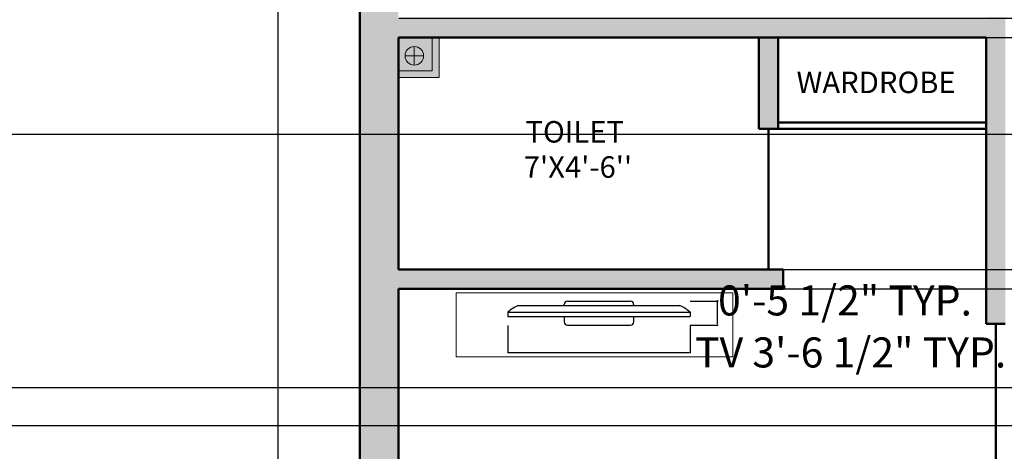
# Model space of a CAD drawing. Units: inches. Extents: x 48 to 822, y -191 to 651.
# Tile 3 of 13: x 429 to 659, y 1 to 101. Entities that reach past the tile are written whole.
import ezdxf

# ---------------------------------------------------------------- set-up
doc = ezdxf.new("R2010")
doc.units = ezdxf.units.IN
doc.header["$MEASUREMENT"] = 0
doc.layers.get('0').update_dxf_attribs({"color": 254})
for name, color, linetype, lineweight in [('A-ANNO-DIMS', 2, 'Continuous', 18), ('A-AREA-IDEN', 7, 'Continuous', 25), ('A-FURN', 8, 'Continuous', 18), ('A-WALL', 7, 'Continuous', 50), ('A-WALL-PATT', 8, 'Continuous', 13)]:
    doc.layers.add(name, color=color, linetype=linetype, lineweight=lineweight)
doc.layers.add('furniture', color=250, linetype='Continuous')
doc.styles.get("Standard").update_dxf_attribs({"font": 'arial.ttf'})
doc.dimstyles.get("Standard").update_dxf_attribs({"dimtxt": 7, "dimasz": 0.18, "dimexe": 0.18, "dimexo": 0.0625, "dimgap": 0.09, "dimtad": 0, "dimtih": 1, "dimtoh": 1, "dimzin": 0, "dimdsep": 46, "dimlunit": 3, "dimtxsty": 'Standard', "dimcen": 0.09, "dimadec": 0, "dimazin": 0, "dimtfac": 1, "dimtofl": 0, "dimtmove": 0, "dimatfit": 3, "dimfxl": 1, "dimtolj": 1, "dimtzin": 0, "dimarcsym": 0})

# ---------------------------------------------------------------- blocks, each defined once
blk = doc.blocks.new('PLASMA-LARGE')
at = {"layer": 'furniture'}
for p, q in [((-7.26, 0), (7.26, 0)), ((-18.61, -1), (18.61, -1)), ((-8, -1), (-8, -0.74)), ((8, -1), (8, -0.74)), ((-21, -2.5), (21, -2.5)), ((-21, -2.5), (-21, -3.5)), ((-21, -3.5), (21, -3.5)), ((-8, -3.5), (-8, -4.76)), ((8, -3.5), (8, -4.76)), ((21, -2.5), (21, -3.5)), ((-7.26, -5.5), (7.26, -5.5))]:
    blk.add_line(p, q, dxfattribs=at)
for centre, radius, start, end in [((-7.26, -0.74), 0.744, 90, 180), ((7.26, -0.74), 0.744, 0, 90), ((-13.97, -11.05), 11.07, 114.7602, 129.4175), ((13.97, -11.05), 11.07, 50.5825, 65.2398), ((-7.26, -4.76), 0.744, 180, 270), ((7.26, -4.76), 0.744, 270, 0)]:
    blk.add_arc(centre, radius, start, end, dxfattribs=at)
blk = doc.blocks.new('*D19')
at = {"layer": 'A-ANNO-DIMS', "color": 0, "lineweight": -2, "transparency": 16777216}
for p, q in [((489.56, 599.69), (489.41, 599.69)), ((489.59, 599.51), (489.59, 243.35)), ((489.59, -120.13), (489.59, 236.02)), ((489.56, -120.31), (489.41, -120.31))]:
    blk.add_line(p, q, dxfattribs=at)
at = {"layer": 'A-ANNO-DIMS', "color": 0, "transparency": 16777216}
for points in [[(489.56, 599.51), (489.62, 599.51), (489.59, 599.69)], [(489.56, -120.13), (489.62, -120.13), (489.59, -120.31)]]:
    blk.add_solid(points, dxfattribs=at)
at = {"layer": 'Defpoints', "color": 0, "transparency": 16777216}
for p in [(489.62, 599.69), (489.59, -120.31), (489.62, -120.31)]:
    blk.add_point(p, dxfattribs=at)
at = {"layer": 'A-ANNO-DIMS', "color": 0, "transparency": 16777216, "insert": (489.59, 239.69), "char_height": 7, "attachment_point": 5}
blk.add_mtext("\\A1;60'", dxfattribs=at)
blk = doc.blocks.new('TV-UNIT')
for p, q in [((14.9, 64.44), (0, 64.44)), ((0, 64.44), (0, 0)), ((14.9, 64.44), (14.9, 0)), ((0, 0), (14.9, 0))]:
    blk.add_line(p, q)
blk = doc.blocks.new('*D34')
at = {"layer": 'A-ANNO-DIMS', "color": 0, "lineweight": -2, "transparency": 16777216}
for p, q in [((543.12, 30.18), (543.12, 23.69)), ((585.6, 30.18), (585.6, 23.69)), ((543.3, 23.87), (585.42, 23.87)), ((585.6, 23.87), (585.78, 23.87))]:
    blk.add_line(p, q, dxfattribs=at)
at = {"layer": 'A-ANNO-DIMS', "color": 0, "transparency": 16777216}
for points in [[(543.3, 23.9), (543.3, 23.84), (543.12, 23.87)], [(585.42, 23.9), (585.42, 23.84), (585.6, 23.87)]]:
    blk.add_solid(points, dxfattribs=at)
at = {"layer": 'Defpoints', "color": 0, "transparency": 16777216}
for p in [(543.12, 30.24), (585.6, 30.24), (585.6, 23.87)]:
    blk.add_point(p, dxfattribs=at)
at = {"layer": 'A-ANNO-DIMS', "color": 0, "transparency": 16777216, "insert": (623.05, 23.87), "char_height": 7, "attachment_point": 5}
blk.add_mtext('\\A1;TV 3\'-6 1/2" TYP.', dxfattribs=at)
blk = doc.blocks.new('*D35')
at = {"layer": 'A-ANNO-DIMS', "color": 0, "lineweight": -2, "transparency": 16777216}
for p, q in [((585.66, 35.8), (592.15, 35.8)), ((591.97, 35.8), (591.97, 35.98)), ((591.97, 35.98), (592.15, 35.98)), ((591.97, 30.42), (591.97, 35.62)), ((585.66, 30.24), (592.15, 30.24))]:
    blk.add_line(p, q, dxfattribs=at)
at = {"layer": 'A-ANNO-DIMS', "color": 0, "transparency": 16777216}
for points in [[(591.94, 35.62), (592, 35.62), (591.97, 35.8)], [(591.94, 30.42), (592, 30.42), (591.97, 30.24)]]:
    blk.add_solid(points, dxfattribs=at)
at = {"layer": 'Defpoints', "color": 0, "transparency": 16777216}
for p in [(585.6, 35.8), (591.97, 35.8), (585.6, 30.24)]:
    blk.add_point(p, dxfattribs=at)
at = {"layer": 'A-ANNO-DIMS', "color": 0, "transparency": 16777216, "insert": (621.73, 35.98), "char_height": 7, "attachment_point": 5}
blk.add_mtext('\\A1;0\'-5 1/2" TYP.', dxfattribs=at)
blk = doc.blocks.new('*D42')
at = {"layer": 'A-ANNO-DIMS', "color": 0, "lineweight": -2, "transparency": 16777216}
for p, q in [((522.85, -26.13), (522.85, -12.54)), ((523.03, -12.72), (525.64, -12.72)), ((612.45, -12.72), (609.84, -12.72)), ((612.63, -26.13), (612.63, -12.54))]:
    blk.add_line(p, q, dxfattribs=at)
at = {"layer": 'A-ANNO-DIMS', "color": 0, "transparency": 16777216}
for points in [[(523.03, -12.69), (523.03, -12.75), (522.85, -12.72)], [(612.45, -12.69), (612.45, -12.75), (612.63, -12.72)]]:
    blk.add_solid(points, dxfattribs=at)
at = {"layer": 'Defpoints', "color": 0, "transparency": 16777216}
for p in [(522.85, -12.72), (522.85, -26.19), (612.63, -26.19)]:
    blk.add_point(p, dxfattribs=at)
at = {"layer": 'A-ANNO-DIMS', "color": 0, "transparency": 16777216, "insert": (567.74, -12.72), "char_height": 7, "attachment_point": 5}
blk.add_mtext('\\A1;DOUBLE BED 7\'-6"', dxfattribs=at)
blk = doc.blocks.new('*D86')
at = {"layer": 'A-ANNO-DIMS', "color": 0, "lineweight": -2, "transparency": 16777216}
for p, q in [((361.01, 74.69), (790.04, 74.69)), ((789.86, 74.51), (789.86, 44.42)), ((789.86, 7.02), (789.86, 37.1)), ((361.01, 6.84), (790.04, 6.84))]:
    blk.add_line(p, q, dxfattribs=at)
at = {"layer": 'A-ANNO-DIMS', "color": 0, "transparency": 16777216}
for points in [[(789.83, 74.51), (789.89, 74.51), (789.86, 74.69)], [(789.83, 7.02), (789.89, 7.02), (789.86, 6.84)]]:
    blk.add_solid(points, dxfattribs=at)
at = {"layer": 'Defpoints', "color": 0, "transparency": 16777216}
for p in [(360.95, 74.69), (360.95, 6.84), (789.86, 6.84)]:
    blk.add_point(p, dxfattribs=at)
at = {"layer": 'A-ANNO-DIMS', "color": 0, "transparency": 16777216, "insert": (789.86, 40.76), "char_height": 7, "attachment_point": 5}
blk.add_mtext('\\A1;5\'-8"', dxfattribs=at)
blk = doc.blocks.new('*D87')
at = {"layer": 'A-ANNO-DIMS', "color": 0, "lineweight": -2, "transparency": 16777216}
for p, q in [((361.01, 6.84), (790.04, 6.84)), ((789.86, 6.66), (789.86, -0.78)), ((789.86, -15.63), (789.86, -8.2)), ((361.01, -15.81), (790.04, -15.81))]:
    blk.add_line(p, q, dxfattribs=at)
at = {"layer": 'A-ANNO-DIMS', "color": 0, "transparency": 16777216}
for points in [[(789.83, 6.66), (789.89, 6.66), (789.86, 6.84)], [(789.83, -15.63), (789.89, -15.63), (789.86, -15.81)]]:
    blk.add_solid(points, dxfattribs=at)
at = {"layer": 'Defpoints', "color": 0, "transparency": 16777216}
for p in [(360.95, 6.84), (360.95, -15.81), (789.86, -15.81)]:
    blk.add_point(p, dxfattribs=at)
at = {"layer": 'A-ANNO-DIMS', "color": 0, "transparency": 16777216, "insert": (789.86, -4.49), "char_height": 7, "attachment_point": 5}
blk.add_mtext('\\A1;1\'-10 1/2"', dxfattribs=at)
blk = doc.blocks.new('*D93')
at = {"layer": 'A-ANNO-DIMS', "color": 0, "lineweight": -2, "transparency": 16777216}
for p, q in [((271.51, 15.7), (790.04, 15.7)), ((789.86, 15.52), (789.86, -8.55)), ((789.86, -39.95), (789.86, -15.88)), ((271.51, -40.13), (790.04, -40.13))]:
    blk.add_line(p, q, dxfattribs=at)
at = {"layer": 'A-ANNO-DIMS', "color": 0, "transparency": 16777216}
for points in [[(789.83, 15.52), (789.89, 15.52), (789.86, 15.7)], [(789.83, -39.95), (789.89, -39.95), (789.86, -40.13)]]:
    blk.add_solid(points, dxfattribs=at)
at = {"layer": 'Defpoints', "color": 0, "transparency": 16777216}
for p in [(271.45, 15.7), (271.45, -40.13), (789.86, -40.13)]:
    blk.add_point(p, dxfattribs=at)
at = {"layer": 'A-ANNO-DIMS', "color": 0, "transparency": 16777216, "insert": (789.86, -12.22), "char_height": 7, "attachment_point": 5}
blk.add_mtext('\\A1;4\'-8"', dxfattribs=at)
blk = doc.blocks.new('*D114')
at = {"layer": 'A-ANNO-DIMS', "color": 0, "lineweight": -2, "transparency": 16777216}
for p, q in [((517.67, 101.69), (790.04, 101.69)), ((789.86, 101.51), (789.86, 97.37)), ((517.67, 97.19), (790.04, 97.19)), ((789.86, 97.01), (789.68, 97.01)), ((789.86, 97.19), (789.86, 97.01))]:
    blk.add_line(p, q, dxfattribs=at)
at = {"layer": 'A-ANNO-DIMS', "color": 0, "transparency": 16777216}
for points in [[(789.83, 101.51), (789.89, 101.51), (789.86, 101.69)], [(789.83, 97.37), (789.89, 97.37), (789.86, 97.19)]]:
    blk.add_solid(points, dxfattribs=at)
at = {"layer": 'Defpoints', "color": 0, "transparency": 16777216}
for p in [(517.61, 101.69), (517.61, 97.19), (789.86, 97.19)]:
    blk.add_point(p, dxfattribs=at)
at = {"layer": 'A-ANNO-DIMS', "color": 0, "transparency": 16777216, "insert": (772.13, 97.01), "char_height": 7, "attachment_point": 5}
blk.add_mtext('\\A1;0\'-4 1/2"', dxfattribs=at)
blk = doc.blocks.new('*D115')
at = {"layer": 'A-ANNO-DIMS', "color": 0, "lineweight": -2, "transparency": 16777216}
for p, q in [((517.67, 97.19), (790.04, 97.19)), ((789.86, 97.01), (789.86, 73.85)), ((789.86, 43.37), (789.86, 66.52)), ((517.67, 43.19), (790.04, 43.19))]:
    blk.add_line(p, q, dxfattribs=at)
at = {"layer": 'A-ANNO-DIMS', "color": 0, "transparency": 16777216}
for points in [[(789.83, 97.01), (789.89, 97.01), (789.86, 97.19)], [(789.83, 43.37), (789.89, 43.37), (789.86, 43.19)]]:
    blk.add_solid(points, dxfattribs=at)
at = {"layer": 'Defpoints', "color": 0, "transparency": 16777216}
for p in [(517.61, 97.19), (517.61, 43.19), (789.86, 43.19)]:
    blk.add_point(p, dxfattribs=at)
at = {"layer": 'A-ANNO-DIMS', "color": 0, "transparency": 16777216, "insert": (789.86, 70.19), "char_height": 7, "attachment_point": 5}
blk.add_mtext('\\A1;4\'-6"', dxfattribs=at)
blk = doc.blocks.new('*D116')
at = {"layer": 'A-ANNO-DIMS', "color": 0, "lineweight": -2, "transparency": 16777216}
for p, q in [((517.67, 43.19), (790.04, 43.19)), ((789.86, 43.01), (789.86, 38.87)), ((517.67, 38.69), (790.04, 38.69)), ((789.86, 38.51), (789.68, 38.51)), ((789.86, 38.69), (789.86, 38.51))]:
    blk.add_line(p, q, dxfattribs=at)
at = {"layer": 'A-ANNO-DIMS', "color": 0, "transparency": 16777216}
for points in [[(789.83, 43.01), (789.89, 43.01), (789.86, 43.19)], [(789.83, 38.87), (789.89, 38.87), (789.86, 38.69)]]:
    blk.add_solid(points, dxfattribs=at)
at = {"layer": 'Defpoints', "color": 0, "transparency": 16777216}
for p in [(517.61, 43.19), (517.61, 38.69), (789.86, 38.69)]:
    blk.add_point(p, dxfattribs=at)
at = {"layer": 'A-ANNO-DIMS', "color": 0, "transparency": 16777216, "insert": (772.13, 38.51), "char_height": 7, "attachment_point": 5}
blk.add_mtext('\\A1;0\'-4 1/2"', dxfattribs=at)
blk = doc.blocks.new('*D117')
at = {"layer": 'A-ANNO-DIMS', "color": 0, "lineweight": -2, "transparency": 16777216}
for p, q in [((517.67, 38.69), (790.04, 38.69)), ((789.86, 38.51), (789.86, -32.65)), ((789.86, -111.13), (789.86, -39.98)), ((517.67, -111.31), (790.04, -111.31))]:
    blk.add_line(p, q, dxfattribs=at)
at = {"layer": 'A-ANNO-DIMS', "color": 0, "transparency": 16777216}
for points in [[(789.83, 38.51), (789.89, 38.51), (789.86, 38.69)], [(789.83, -111.13), (789.89, -111.13), (789.86, -111.31)]]:
    blk.add_solid(points, dxfattribs=at)
at = {"layer": 'Defpoints', "color": 0, "transparency": 16777216}
for p in [(517.61, 38.69), (517.61, -111.31), (789.86, -111.31)]:
    blk.add_point(p, dxfattribs=at)
at = {"layer": 'A-ANNO-DIMS', "color": 0, "transparency": 16777216, "insert": (789.86, -36.31), "char_height": 7, "attachment_point": 5}
blk.add_mtext('\\A1;12\'-6"', dxfattribs=at)

msp = doc.modelspace()

# ---------------------------------------------------------------- hatches: boundary and pattern name
at = {"layer": 'A-FURN'}
h = msp.add_hatch(color=256, dxfattribs=at)
h.dxf.hatch_style = 1
h.paths.add_polyline_path([(527.093, 97.187), (525.459, 97.187), (525.459, 89.426), (517.61, 89.426), (517.61, 87.871), (527.093, 87.871)])
h.paths.add_polyline_path([(525.459, 97.187), (517.61, 97.187), (517.61, 89.426), (525.459, 89.426)], flags=17)
h.paths.add_polyline_path([(519.148, 92.943, -1), (523.47, 92.943, -1)], flags=16)
h = msp.add_hatch(color=256, dxfattribs=at)
h.dxf.hatch_style = 1
h.paths.add_polyline_path([(521.309, 95.105, 0.4142136), (519.148, 92.943), (521.309, 92.943)])
h.paths.add_polyline_path([(521.309, 95.105), (521.309, 92.943), (523.47, 92.943, 0.4142136)])
h.paths.add_polyline_path([(523.47, 92.943), (521.309, 92.943), (521.309, 90.782, 0.4142136)])
h.paths.add_polyline_path([(521.309, 92.943), (519.148, 92.943, 0.4142136), (521.309, 90.782)])
at = {"layer": 'A-WALL-PATT'}
h = msp.add_hatch(color=256, dxfattribs=at)
h.dxf.hatch_style = 1
h.paths.add_polyline_path([(614.11, 432.437), (609.61, 432.437), (609.61, 376.187), (535.284, 376.187), (535.284, 371.687), (547.61, 371.687), (547.61, 359.12), (552.11, 359.12), (552.11, 371.687), (609.61, 371.687), (609.61, 335.687), (614.11, 335.687)], flags=17)
h.paths.add_polyline_path([(614.11, 434.687), (609.61, 434.687), (609.61, 432.437), (614.11, 432.437)], flags=17)
h.paths.add_polyline_path([(573.934, 434.687), (517.61, 434.687), (517.61, 590.687), (650.61, 590.687), (650.61, 585.522), (655.11, 585.522), (655.11, 590.687), (739.61, 590.687), (739.61, 548.687), (655.11, 548.687), (655.11, 550.72), (650.61, 550.72), (650.61, 458.608), (655.11, 458.608), (655.11, 544.187), (739.61, 544.187), (739.61, 434.541), (650.61, 434.541), (650.61, 430.041), (739.61, 430.041), (739.61, -16.844), (729.973, -16.844), (729.973, -21.344), (748.61, -21.344), (748.61, 599.687), (508.61, 599.687), (508.61, -120.313), (543.114, -120.313), (543.114, -111.313), (517.61, -111.313), (517.61, 38.687), (607.29, 38.687), (607.29, 43.187), (517.61, 43.187), (517.61, 97.187), (654.61, 97.187), (654.61, 30.562), (659.11, 30.562), (659.11, 101.895), (654.61, 101.895), (654.61, 101.687), (517.61, 101.687), (517.61, 221.687), (654.61, 221.687), (654.61, 218.066), (659.11, 218.066), (659.11, 226.187), (517.61, 226.187), (517.61, 295.187), (614.11, 295.187), (648.087, 295.187), (661.07, 295.187), (661.07, 299.687), (614.11, 299.687), (552.11, 299.687), (552.11, 341.37), (547.61, 341.37), (547.61, 299.687), (517.61, 299.687), (517.61, 371.687), (517.534, 371.687), (517.534, 376.187), (517.61, 430.187), (573.934, 430.187)])
h.paths.add_polyline_path([(659.11, -87.328), (654.61, -87.328), (654.61, -111.313), (598.94, -111.313), (598.94, -120.313), (659.11, -120.313)], flags=0)
h.paths.add_polyline_path([(671.266, -16.844), (659.11, -16.844), (659.11, -12.05), (654.61, -12.05), (654.61, -31.502), (659.11, -31.502), (659.11, -21.344), (671.266, -21.344)], flags=17)
h.paths.add_polyline_path([(606.11, 97.187), (601.61, 97.187), (601.61, 75.902), (606.11, 75.902)], flags=17)
h.paths.add_polyline_path([(659.11, 169.875), (654.61, 169.875), (654.61, 157.721), (659.11, 157.721)], flags=17)

# ---------------------------------------------------------------- linework, layer by layer
at = {"layer": 'A-FURN'}
for p, q in [((525.459, 89.426), (525.459, 97.187)), ((527.093, 87.871), (527.093, 97.187)), ((521.309, 95.105), (521.309, 90.782)), ((519.148, 92.943), (523.47, 92.943)), ((517.61, 89.426), (517.61, 89.426)), ((517.61, 89.426), (525.459, 89.426)), ((517.61, 87.871), (527.093, 87.871))]:
    msp.add_line(p, q, dxfattribs=at)
msp.add_circle((521.309, 92.943), 2.161, dxfattribs=at)
at = {"layer": 'A-WALL'}
for p, q in [((508.61, -120.313), (508.61, 599.687)), ((654.61, 97.187), (517.61, 97.187)), ((517.61, 43.187), (517.61, 97.187)), ((601.61, 75.902), (601.61, 97.187)), ((606.11, 75.902), (606.11, 97.187)), ((654.61, 30.562), (654.61, 97.187)), ((606.11, 75.902), (601.61, 75.902)), ((603.86, 75.902), (603.86, 43.187)), ((654.61, 77.439), (606.11, 77.439)), ((606.11, 75.902), (654.61, 75.902)), ((607.29, 43.187), (517.61, 43.187)), ((607.29, 43.187), (607.29, 38.687)), ((517.61, -111.313), (517.61, 38.687)), ((607.29, 38.687), (517.61, 38.687)), ((654.61, 30.562), (659.11, 30.562)), ((656.86, 30.562), (656.86, -12.05))]:
    msp.add_line(p, q, dxfattribs=at)

# ---------------------------------------------------------------- block references
at = {"layer": 'A-FURN', "rotation": 270.0000000000002}
msp.add_blockref('TV-UNIT', (531.097, 37.751), dxfattribs=at)
at = {"layer": 'A-FURN', "xscale": 1.011294184530666, "yscale": 1.011294184530666, "zscale": 1.011294184530666}
msp.add_blockref('PLASMA-LARGE', (564.359, 35.801), dxfattribs=at)

# ---------------------------------------------------------------- texts
at = {"layer": 'A-AREA-IDEN'}
for s, p in [('WARDROBE', (610.434, 84.249)), ('TOILET', (547.225, 72.739)), ("7'X4'-6''", (546.821, 64.535))]:
    msp.add_text(s, height=5.0075, dxfattribs=at).set_placement(p)

# ---------------------------------------------------------------- dimensions: what is measured, and where the dimension line sits
at = {"layer": 'A-ANNO-DIMS'}
for base, p1, p2, override, picture, middle in [((489.59, -120.313), (489.619, 599.687), (489.619, -120.313), {"dimclrd": 0, "dimclre": 0, "dimclrt": 0}, '*D19', (489.59, 239.687)), ((789.86, 97.187), (517.61, 101.687), (517.61, 97.187), {"dimdec": 1, "dimlfac": 1, "dimrnd": 0, "dimzin": 1, "dimdsep": 46, "dimlunit": 4, "dimfrac": 2}, '*D114', (772.131, 97.007)), ((789.86, 43.187), (517.61, 97.187), (517.61, 43.187), {"dimdec": 1, "dimlfac": 1, "dimrnd": 0, "dimzin": 1, "dimdsep": 46, "dimlunit": 4, "dimfrac": 2}, '*D115', (789.86, 70.187)), ((789.86, 6.835), (360.951, 74.687), (360.951, 6.835), {"dimdec": 1, "dimlfac": 1, "dimrnd": 0, "dimzin": 1, "dimdsep": 46, "dimlunit": 4, "dimfrac": 2}, '*D86', (789.86, 40.761)), ((789.86, 38.687), (517.61, 43.187), (517.61, 38.687), {"dimdec": 1, "dimlfac": 1, "dimrnd": 0, "dimzin": 1, "dimdsep": 46, "dimlunit": 4, "dimfrac": 2}, '*D116', (772.131, 38.507)), ((789.86, -111.313), (517.61, 38.687), (517.61, -111.313), {"dimdec": 1, "dimlfac": 1, "dimrnd": 0, "dimzin": 1, "dimdsep": 46, "dimlunit": 4, "dimfrac": 2}, '*D117', (789.86, -36.313)), ((789.86, -40.13), (271.451, 15.696), (271.451, -40.13), {"dimdec": 1, "dimlfac": 1, "dimrnd": 0, "dimzin": 1, "dimdsep": 46, "dimlunit": 4, "dimfrac": 2}, '*D93', (789.86, -12.217)), ((789.86, -15.813), (360.951, 6.835), (360.951, -15.813), {"dimdec": 1, "dimlfac": 1, "dimrnd": 0, "dimzin": 1, "dimdsep": 46, "dimlunit": 4, "dimfrac": 2}, '*D87', (789.86, -4.489))]:
    dim = msp.add_linear_dim(base=base, p1=p1, p2=p2, angle=90, dimstyle='Standard', override=override, dxfattribs=at)
    dim.commit()
    dim.dimension.update_dxf_attribs({"geometry": picture, "text_midpoint": middle})
for base, p1, p2, angle, text, picture, middle in [((591.967, 35.801), (585.596, 30.239), (585.596, 35.801), 90, '<> TYP.', '*D35', (621.727, 35.981)), ((522.854, -12.724), (612.63, -26.191), (522.854, -26.191), 180, 'DOUBLE BED <>', '*D42', (567.742, -12.724))]:
    dim = msp.add_linear_dim(base=base, p1=p1, p2=p2, angle=angle, text=text, dimstyle='Standard', override={"dimdec": 1, "dimlfac": 1, "dimrnd": 0, "dimzin": 1, "dimdsep": 46, "dimlunit": 4, "dimfrac": 2}, dxfattribs=at)
    dim.commit()
    dim.dimension.update_dxf_attribs({"geometry": picture, "text_midpoint": middle})
dim = msp.add_linear_dim(base=(585.596, 23.868), p1=(543.121, 30.239), p2=(585.596, 30.239), text='TV <> TYP.', dimstyle='Standard', override={"dimdec": 1, "dimlfac": 1, "dimrnd": 0, "dimzin": 1, "dimdsep": 46, "dimlunit": 4, "dimfrac": 2}, dxfattribs=at)
dim.commit()
dim.dimension.update_dxf_attribs({"geometry": '*D34', "text_midpoint": (623.05, 23.868)})

doc.saveas('drawing.dxf')
